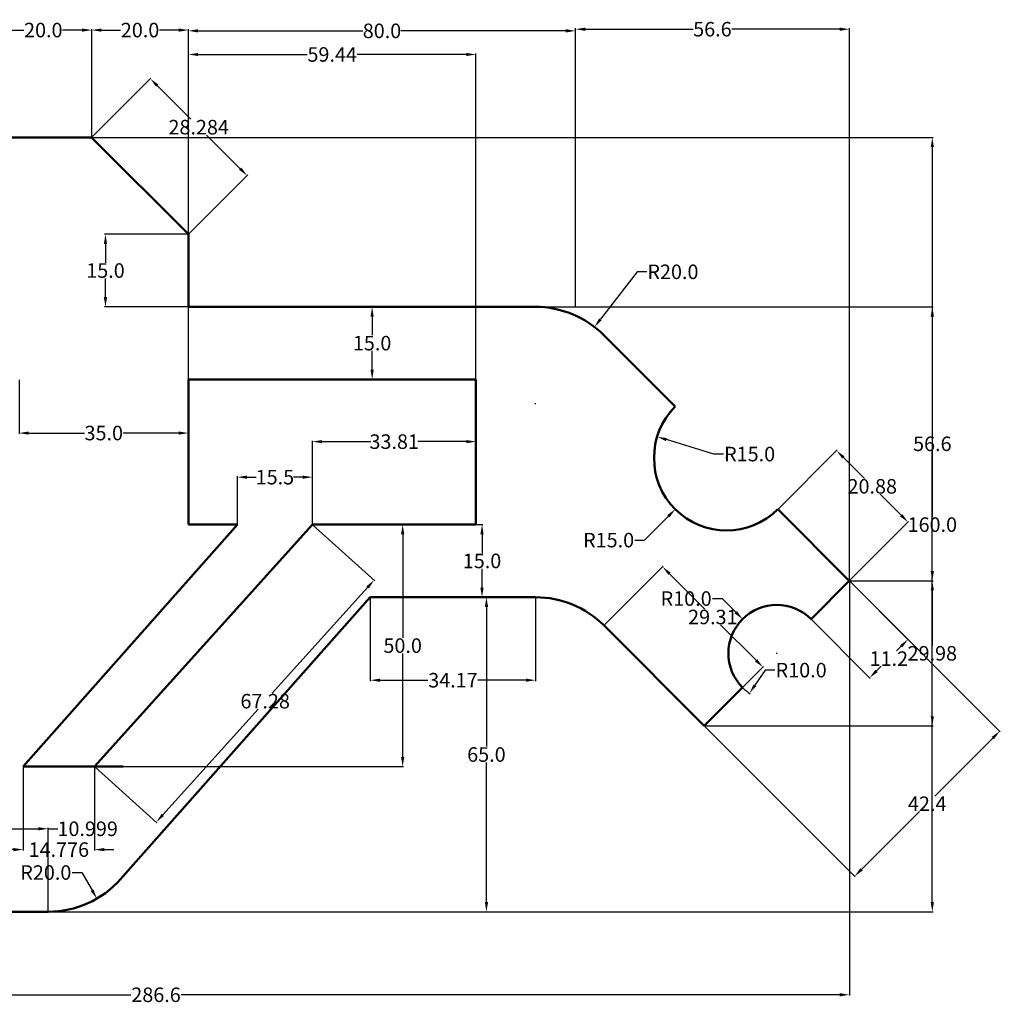
# Model space of a CAD drawing. Units: inches. Extents: x 142 to 482, y 54 to 269.
# Tile 2 of 2: x 279 to 482, y 54 to 258. Entities that reach past the tile are written whole.
import ezdxf

# ---------------------------------------------------------------- set-up
doc = ezdxf.new("R2010")
doc.units = ezdxf.units.IN
doc.header["$MEASUREMENT"] = 0
doc.layers.add('M-DIMS', color=2, linetype='Continuous', lineweight=25)
doc.layers.add('M-OUTL', color=7, linetype='Continuous', lineweight=50)
doc.styles.get("Standard").update_dxf_attribs({"font": 'arial.ttf'})
doc.dimstyles.get("Standard").update_dxf_attribs({"dimtxt": 3, "dimasz": 2, "dimexe": 0.18, "dimexo": 0.0625, "dimgap": 0.09, "dimtad": 0, "dimtih": 1, "dimtoh": 1, "dimdec": 1, "dimzin": 0, "dimdsep": 46, "dimtxsty": 'Standard', "dimcen": 0.09, "dimclrd": 1, "dimclre": 1, "dimadec": 0, "dimazin": 0, "dimtfac": 1, "dimtdec": 1, "dimtofl": 0, "dimtmove": 0, "dimatfit": 3, "dimfxl": 1, "dimtolj": 1, "dimtzin": 0, "dimarcsym": 0})

# ---------------------------------------------------------------- blocks, each defined once
blk = doc.blocks.new('*D9')
at = {"layer": 'Defpoints', "color": 0, "transparency": 16777216}
for p in [(293.74, 255.73), (273.74, 233.54), (293.74, 233.54)]:
    blk.add_point(p, dxfattribs=at)
at = {"layer": 'M-DIMS', "color": 0, "lineweight": -2, "transparency": 16777216}
for p, q in [((273.74, 233.6), (273.74, 255.91)), ((275.74, 255.73), (279.73, 255.73)), ((291.74, 255.73), (287.74, 255.73)), ((293.74, 233.6), (293.74, 255.91))]:
    blk.add_line(p, q, dxfattribs=at)
at = {"layer": 'M-DIMS', "color": 0, "transparency": 16777216}
for points in [[(275.74, 256.06), (275.74, 255.39), (273.74, 255.73)], [(291.74, 256.06), (291.74, 255.39), (293.74, 255.73)]]:
    blk.add_solid(points, dxfattribs=at)
at = {"layer": 'M-DIMS', "color": 0, "transparency": 16777216, "insert": (283.74, 255.73), "char_height": 3, "attachment_point": 5}
blk.add_mtext('\\A1;20.0', dxfattribs=at)
blk = doc.blocks.new('*D10')
at = {"layer": 'Defpoints', "color": 0, "transparency": 16777216}
for p in [(293.74, 255.73), (293.74, 233.54), (313.74, 213.54)]:
    blk.add_point(p, dxfattribs=at)
at = {"layer": 'M-DIMS', "color": 0, "lineweight": -2, "transparency": 16777216}
for p, q in [((293.74, 233.6), (293.74, 255.91)), ((295.74, 255.73), (299.73, 255.73)), ((311.74, 255.73), (307.74, 255.73)), ((313.74, 213.6), (313.74, 255.91))]:
    blk.add_line(p, q, dxfattribs=at)
at = {"layer": 'M-DIMS', "color": 0, "transparency": 16777216}
for points in [[(295.74, 256.06), (295.74, 255.39), (293.74, 255.73)], [(311.74, 256.06), (311.74, 255.39), (313.74, 255.73)]]:
    blk.add_solid(points, dxfattribs=at)
at = {"layer": 'M-DIMS', "color": 0, "transparency": 16777216, "insert": (303.74, 255.73), "char_height": 3, "attachment_point": 5}
blk.add_mtext('\\A1;20.0', dxfattribs=at)
blk = doc.blocks.new('*D11')
at = {"layer": 'Defpoints', "color": 0, "transparency": 16777216}
for p in [(351.7, 198.54), (336.38, 183.54), (351.7, 183.54)]:
    blk.add_point(p, dxfattribs=at)
at = {"layer": 'M-DIMS', "color": 0, "lineweight": -2, "transparency": 16777216}
for p, q in [((351.76, 198.54), (351.88, 198.54)), ((351.7, 196.54), (351.7, 192.66)), ((351.7, 185.54), (351.7, 189.42)), ((336.44, 183.54), (351.88, 183.54))]:
    blk.add_line(p, q, dxfattribs=at)
at = {"layer": 'M-DIMS', "color": 0, "transparency": 16777216}
for points in [[(351.37, 196.54), (352.03, 196.54), (351.7, 198.54)], [(351.37, 185.54), (352.03, 185.54), (351.7, 183.54)]]:
    blk.add_solid(points, dxfattribs=at)
at = {"layer": 'M-DIMS', "color": 0, "transparency": 16777216, "insert": (351.7, 191.04), "char_height": 3, "attachment_point": 5}
blk.add_mtext('\\A1;15.0', dxfattribs=at)
blk = doc.blocks.new('*D12')
at = {"layer": 'Defpoints', "color": 0, "transparency": 16777216}
for p in [(344.57, 153.54), (358.02, 153.54), (300.27, 103.54)]:
    blk.add_point(p, dxfattribs=at)
at = {"layer": 'M-DIMS', "color": 0, "lineweight": -2, "transparency": 16777216}
for p, q in [((344.63, 153.54), (358.2, 153.54)), ((358.02, 151.54), (358.02, 130.16)), ((358.02, 105.54), (358.02, 126.92)), ((300.34, 103.54), (358.2, 103.54))]:
    blk.add_line(p, q, dxfattribs=at)
at = {"layer": 'M-DIMS', "color": 0, "transparency": 16777216}
for points in [[(357.68, 151.54), (358.35, 151.54), (358.02, 153.54)], [(357.68, 105.54), (358.35, 105.54), (358.02, 103.54)]]:
    blk.add_solid(points, dxfattribs=at)
at = {"layer": 'M-DIMS', "color": 0, "transparency": 16777216, "insert": (358.02, 128.54), "char_height": 3, "attachment_point": 5}
blk.add_mtext('\\A1;50.0', dxfattribs=at)
blk = doc.blocks.new('*D13')
at = {"layer": 'Defpoints', "color": 0, "transparency": 16777216}
for p in [(372.53, 138.54), (375.33, 138.54), (284.73, 73.54)]:
    blk.add_point(p, dxfattribs=at)
at = {"layer": 'M-DIMS', "color": 0, "lineweight": -2, "transparency": 16777216}
for p, q in [((372.59, 138.54), (375.51, 138.54)), ((375.33, 136.54), (375.33, 107.66)), ((375.33, 75.54), (375.33, 104.42)), ((284.8, 73.54), (375.51, 73.54))]:
    blk.add_line(p, q, dxfattribs=at)
at = {"layer": 'M-DIMS', "color": 0, "transparency": 16777216}
for points in [[(375, 136.54), (375.67, 136.54), (375.33, 138.54)], [(375, 75.54), (375.67, 75.54), (375.33, 73.54)]]:
    blk.add_solid(points, dxfattribs=at)
at = {"layer": 'M-DIMS', "color": 0, "transparency": 16777216, "insert": (375.33, 106.04), "char_height": 3, "attachment_point": 5}
blk.add_mtext('\\A1;65.0', dxfattribs=at)
blk = doc.blocks.new('*D14')
at = {"layer": 'Defpoints', "color": 0, "transparency": 16777216}
for p in [(284.73, 93.54), (294.82, 76.27)]:
    blk.add_point(p, dxfattribs=at)
at = {"layer": 'M-DIMS', "color": 0, "lineweight": -2, "transparency": 16777216}
for p, q in [((289.68, 81.65), (291.68, 81.65)), ((291.68, 81.65), (293.81, 77.99))]:
    blk.add_line(p, q, dxfattribs=at)
at = {"layer": 'M-DIMS', "color": 0, "transparency": 16777216}
blk.add_solid([(294.1, 78.16), (293.52, 77.82), (294.82, 76.27)], dxfattribs=at)
at = {"layer": 'M-DIMS', "color": 0, "transparency": 16777216, "insert": (284.26, 81.65), "char_height": 3, "attachment_point": 5}
blk.add_mtext('\\A1;R20.0', dxfattribs=at)
blk = doc.blocks.new('*D15')
at = {"layer": 'Defpoints', "color": 0, "transparency": 16777216}
for p in [(393.74, 255.91), (393.74, 198.54), (450.34, 141.94)]:
    blk.add_point(p, dxfattribs=at)
at = {"layer": 'M-DIMS', "color": 0, "lineweight": -2, "transparency": 16777216}
for p, q in [((393.74, 198.6), (393.74, 256.09)), ((395.74, 255.91), (418.05, 255.91)), ((448.34, 255.91), (426.02, 255.91)), ((450.34, 142), (450.34, 256.09))]:
    blk.add_line(p, q, dxfattribs=at)
at = {"layer": 'M-DIMS', "color": 0, "transparency": 16777216}
for points in [[(395.74, 256.24), (395.74, 255.57), (393.74, 255.91)], [(448.34, 256.24), (448.34, 255.57), (450.34, 255.91)]]:
    blk.add_solid(points, dxfattribs=at)
at = {"layer": 'M-DIMS', "color": 0, "transparency": 16777216, "insert": (422.04, 255.91), "char_height": 3, "attachment_point": 5}
blk.add_mtext('\\A1;56.6', dxfattribs=at)
blk = doc.blocks.new('*D16')
at = {"layer": 'Defpoints', "color": 0, "transparency": 16777216}
for p in [(450.34, 141.94), (420.35, 111.96), (451.43, 80.88)]:
    blk.add_point(p, dxfattribs=at)
at = {"layer": 'M-DIMS', "color": 0, "lineweight": -2, "transparency": 16777216}
for p, q in [((450.38, 141.89), (481.54, 110.73)), ((420.4, 111.91), (451.56, 80.75)), ((480, 109.44), (468.02, 97.46)), ((452.85, 82.29), (464.83, 94.27))]:
    blk.add_line(p, q, dxfattribs=at)
at = {"layer": 'M-DIMS', "color": 0, "transparency": 16777216}
for points in [[(479.77, 109.68), (480.24, 109.21), (481.42, 110.86)], [(452.61, 82.53), (453.08, 82.06), (451.43, 80.88)]]:
    blk.add_solid(points, dxfattribs=at)
at = {"layer": 'M-DIMS', "color": 0, "transparency": 16777216, "insert": (466.43, 95.87), "char_height": 3, "attachment_point": 5}
blk.add_mtext('\\A1;42.4', dxfattribs=at)
blk = doc.blocks.new('*D17')
at = {"layer": 'Defpoints', "color": 0, "transparency": 16777216}
for p in [(397.67, 194.38), (385.45, 178.54)]:
    blk.add_point(p, dxfattribs=at)
at = {"layer": 'M-DIMS', "color": 0, "lineweight": -2, "transparency": 16777216}
for p, q in [((406.46, 205.78), (398.89, 195.96)), ((408.46, 205.78), (406.46, 205.78)), ((385.36, 178.54), (385.54, 178.54)), ((385.45, 178.45), (385.45, 178.63))]:
    blk.add_line(p, q, dxfattribs=at)
at = {"layer": 'M-DIMS', "color": 0, "transparency": 16777216}
blk.add_solid([(398.62, 196.16), (399.15, 195.76), (397.67, 194.38)], dxfattribs=at)
at = {"layer": 'M-DIMS', "color": 0, "transparency": 16777216, "insert": (413.88, 205.78), "char_height": 3, "attachment_point": 5}
blk.add_mtext('\\A1;R20.0', dxfattribs=at)
blk = doc.blocks.new('*D18')
at = {"layer": 'Defpoints', "color": 0, "transparency": 16777216}
for p in [(373.17, 153.54), (374.42, 138.54), (374.42, 138.54)]:
    blk.add_point(p, dxfattribs=at)
at = {"layer": 'M-DIMS', "color": 0, "lineweight": -2, "transparency": 16777216}
for p, q in [((373.23, 153.54), (374.6, 153.54)), ((374.42, 151.54), (374.42, 147.66)), ((374.42, 140.54), (374.42, 144.42)), ((374.48, 138.54), (374.6, 138.54))]:
    blk.add_line(p, q, dxfattribs=at)
at = {"layer": 'M-DIMS', "color": 0, "transparency": 16777216}
for points in [[(374.08, 151.54), (374.75, 151.54), (374.42, 153.54)], [(374.08, 140.54), (374.75, 140.54), (374.42, 138.54)]]:
    blk.add_solid(points, dxfattribs=at)
at = {"layer": 'M-DIMS', "color": 0, "transparency": 16777216, "insert": (374.42, 146.04), "char_height": 3, "attachment_point": 5}
blk.add_mtext('\\A1;15.0', dxfattribs=at)
blk = doc.blocks.new('*D19')
at = {"layer": 'Defpoints', "color": 0, "transparency": 16777216}
for p in [(339.36, 163.35), (323.86, 153.54), (339.36, 153.54)]:
    blk.add_point(p, dxfattribs=at)
at = {"layer": 'M-DIMS', "color": 0, "lineweight": -2, "transparency": 16777216}
for p, q in [((323.86, 153.6), (323.86, 163.53)), ((325.86, 163.35), (327.76, 163.35)), ((337.36, 163.35), (335.47, 163.35)), ((339.36, 153.6), (339.36, 163.53))]:
    blk.add_line(p, q, dxfattribs=at)
at = {"layer": 'M-DIMS', "color": 0, "transparency": 16777216}
for points in [[(325.86, 163.68), (325.86, 163.01), (323.86, 163.35)], [(337.36, 163.68), (337.36, 163.01), (339.36, 163.35)]]:
    blk.add_solid(points, dxfattribs=at)
at = {"layer": 'M-DIMS', "color": 0, "transparency": 16777216, "insert": (331.61, 163.35), "char_height": 3, "attachment_point": 5}
blk.add_mtext('\\A1;15.5', dxfattribs=at)
blk = doc.blocks.new('*D20')
at = {"layer": 'Defpoints', "color": 0, "transparency": 16777216}
for p in [(435.35, 126.95), (429.7, 118.69)]:
    blk.add_point(p, dxfattribs=at)
at = {"layer": 'M-DIMS', "color": 0, "lineweight": -2, "transparency": 16777216}
for p, q in [((432.97, 123.47), (430.83, 120.34)), ((434.97, 123.47), (432.97, 123.47))]:
    blk.add_line(p, q, dxfattribs=at)
blk.add_arc((435.35, 126.95), 10, 225.3581, 236.6689, dxfattribs=at)
at = {"layer": 'M-DIMS', "color": 0, "transparency": 16777216}
blk.add_solid([(430.55, 120.53), (431.1, 120.16), (429.7, 118.69)], dxfattribs=at)
at = {"layer": 'M-DIMS', "color": 0, "transparency": 16777216, "insert": (440.38, 123.47), "char_height": 3, "attachment_point": 5}
blk.add_mtext('\\A1;R10.0', dxfattribs=at)
blk = doc.blocks.new('*D21')
at = {"layer": 'Defpoints', "color": 0, "transparency": 16777216}
for p in [(410.62, 171.68), (424.96, 167.31)]:
    blk.add_point(p, dxfattribs=at)
at = {"layer": 'M-DIMS', "color": 0, "lineweight": -2, "transparency": 16777216}
for p, q in [((422.31, 168.12), (412.53, 171.1)), ((424.31, 168.12), (422.31, 168.12))]:
    blk.add_line(p, q, dxfattribs=at)
at = {"layer": 'M-DIMS', "color": 0, "transparency": 16777216}
blk.add_solid([(412.63, 171.42), (412.43, 170.78), (410.62, 171.68)], dxfattribs=at)
at = {"layer": 'M-DIMS', "color": 0, "transparency": 16777216, "insert": (429.73, 168.12), "char_height": 3, "attachment_point": 5}
blk.add_mtext('\\A1;R15.0', dxfattribs=at)
blk = doc.blocks.new('*D25')
at = {"layer": 'Defpoints', "color": 0, "transparency": 16777216}
for p in [(393.74, 255.57), (313.74, 213.54), (393.74, 198.54)]:
    blk.add_point(p, dxfattribs=at)
at = {"layer": 'M-DIMS', "color": 0, "lineweight": -2, "transparency": 16777216}
for p, q in [((313.74, 213.6), (313.74, 255.75)), ((315.74, 255.57), (349.75, 255.57)), ((391.74, 255.57), (357.72, 255.57)), ((393.74, 198.6), (393.74, 255.75))]:
    blk.add_line(p, q, dxfattribs=at)
at = {"layer": 'M-DIMS', "color": 0, "transparency": 16777216}
for points in [[(315.74, 255.91), (315.74, 255.24), (313.74, 255.57)], [(391.74, 255.91), (391.74, 255.24), (393.74, 255.57)]]:
    blk.add_solid(points, dxfattribs=at)
at = {"layer": 'M-DIMS', "color": 0, "transparency": 16777216, "insert": (353.74, 255.57), "char_height": 3, "attachment_point": 5}
blk.add_mtext('\\A1;80.0', dxfattribs=at)
blk = doc.blocks.new('*D26')
at = {"layer": 'Defpoints', "color": 0, "transparency": 16777216}
for p in [(278.74, 183.54), (313.74, 183.54), (313.74, 172.46)]:
    blk.add_point(p, dxfattribs=at)
at = {"layer": 'M-DIMS', "color": 0, "lineweight": -2, "transparency": 16777216}
for p, q in [((278.74, 183.48), (278.74, 172.28)), ((313.74, 183.48), (313.74, 172.28)), ((280.74, 172.46), (292.26, 172.46)), ((311.74, 172.46), (300.22, 172.46))]:
    blk.add_line(p, q, dxfattribs=at)
at = {"layer": 'M-DIMS', "color": 0, "transparency": 16777216}
for points in [[(280.74, 172.79), (280.74, 172.13), (278.74, 172.46)], [(311.74, 172.79), (311.74, 172.13), (313.74, 172.46)]]:
    blk.add_solid(points, dxfattribs=at)
at = {"layer": 'M-DIMS', "color": 0, "transparency": 16777216, "insert": (296.24, 172.46), "char_height": 3, "attachment_point": 5}
blk.add_mtext('\\A1;35.0', dxfattribs=at)
blk = doc.blocks.new('*D27')
at = {"layer": 'Defpoints', "color": 0, "transparency": 16777216}
for p in [(450.34, 141.94), (163.74, 93.54), (450.34, 56.39)]:
    blk.add_point(p, dxfattribs=at)
at = {"layer": 'M-DIMS', "color": 1, "lineweight": -2, "transparency": 16777216}
for p, q in [((450.34, 141.88), (450.34, 56.21)), ((163.74, 93.48), (163.74, 56.21)), ((165.74, 56.39), (301.86, 56.39)), ((448.34, 56.39), (312.21, 56.39))]:
    blk.add_line(p, q, dxfattribs=at)
at = {"layer": 'M-DIMS', "color": 1, "transparency": 16777216}
for points in [[(165.74, 56.72), (165.74, 56.06), (163.74, 56.39)], [(448.34, 56.72), (448.34, 56.06), (450.34, 56.39)]]:
    blk.add_solid(points, dxfattribs=at)
at = {"layer": 'M-DIMS', "color": 0, "transparency": 16777216, "insert": (307.04, 56.39), "char_height": 3, "attachment_point": 5}
blk.add_mtext('\\A1;286.6', dxfattribs=at)
blk = doc.blocks.new('*D28')
at = {"layer": 'Defpoints', "color": 0, "transparency": 16777216}
for p in [(293.74, 233.54), (467.49, 233.54), (284.73, 73.54)]:
    blk.add_point(p, dxfattribs=at)
at = {"layer": 'M-DIMS', "color": 1, "lineweight": -2, "transparency": 16777216}
for p, q in [((293.8, 233.54), (467.67, 233.54)), ((467.49, 231.54), (467.49, 155.16)), ((467.49, 75.54), (467.49, 151.92)), ((284.8, 73.54), (467.67, 73.54))]:
    blk.add_line(p, q, dxfattribs=at)
at = {"layer": 'M-DIMS', "color": 1, "transparency": 16777216}
for points in [[(467.15, 231.54), (467.82, 231.54), (467.49, 233.54)], [(467.15, 75.54), (467.82, 75.54), (467.49, 73.54)]]:
    blk.add_solid(points, dxfattribs=at)
at = {"layer": 'M-DIMS', "color": 0, "transparency": 16777216, "insert": (467.49, 153.54), "char_height": 3, "attachment_point": 5}
blk.add_mtext('\\A1;160.0', dxfattribs=at)
blk = doc.blocks.new('*D30')
at = {"layer": 'Defpoints', "color": 0, "transparency": 16777216}
for p in [(373.17, 250.69), (313.74, 183.54), (373.17, 183.54)]:
    blk.add_point(p, dxfattribs=at)
at = {"layer": 'M-DIMS', "color": 1, "lineweight": -2, "transparency": 16777216}
for p, q in [((313.74, 183.6), (313.74, 250.87)), ((315.74, 250.69), (338.31, 250.69)), ((371.17, 250.69), (348.6, 250.69)), ((373.17, 183.6), (373.17, 250.87))]:
    blk.add_line(p, q, dxfattribs=at)
at = {"layer": 'M-DIMS', "color": 1, "transparency": 16777216}
for points in [[(315.74, 251.02), (315.74, 250.36), (313.74, 250.69)], [(371.17, 251.02), (371.17, 250.36), (373.17, 250.69)]]:
    blk.add_solid(points, dxfattribs=at)
at = {"layer": 'M-DIMS', "color": 0, "transparency": 16777216, "insert": (343.45, 250.69), "char_height": 3, "attachment_point": 5}
blk.add_mtext('\\A1;59.44', dxfattribs=at)
blk = doc.blocks.new('*D31')
at = {"layer": 'Defpoints', "color": 0, "transparency": 16777216}
for p in [(296.59, 213.54), (313.74, 213.54), (313.74, 198.54)]:
    blk.add_point(p, dxfattribs=at)
at = {"layer": 'M-DIMS', "color": 1, "lineweight": -2, "transparency": 16777216}
for p, q in [((313.67, 213.54), (296.41, 213.54)), ((296.59, 211.54), (296.59, 207.66)), ((296.59, 200.54), (296.59, 204.42)), ((313.67, 198.54), (296.41, 198.54))]:
    blk.add_line(p, q, dxfattribs=at)
at = {"layer": 'M-DIMS', "color": 1, "transparency": 16777216}
for points in [[(296.25, 211.54), (296.92, 211.54), (296.59, 213.54)], [(296.25, 200.54), (296.92, 200.54), (296.59, 198.54)]]:
    blk.add_solid(points, dxfattribs=at)
at = {"layer": 'M-DIMS', "color": 0, "transparency": 16777216, "insert": (296.59, 206.04), "char_height": 3, "attachment_point": 5}
blk.add_mtext('\\A1;15.0', dxfattribs=at)
blk = doc.blocks.new('*D32')
at = {"layer": 'Defpoints', "color": 0, "transparency": 16777216}
for p in [(373.17, 170.69), (339.36, 153.54), (373.17, 153.54)]:
    blk.add_point(p, dxfattribs=at)
at = {"layer": 'M-DIMS', "color": 1, "lineweight": -2, "transparency": 16777216}
for p, q in [((339.36, 153.6), (339.36, 170.87)), ((341.36, 170.69), (351.41, 170.69)), ((371.17, 170.69), (361.13, 170.69)), ((373.17, 153.6), (373.17, 170.87))]:
    blk.add_line(p, q, dxfattribs=at)
at = {"layer": 'M-DIMS', "color": 1, "transparency": 16777216}
for points in [[(341.36, 171.02), (341.36, 170.36), (339.36, 170.69)], [(371.17, 171.02), (371.17, 170.36), (373.17, 170.69)]]:
    blk.add_solid(points, dxfattribs=at)
at = {"layer": 'M-DIMS', "color": 0, "transparency": 16777216, "insert": (356.27, 170.69), "char_height": 3, "attachment_point": 5}
blk.add_mtext('\\A1;33.81', dxfattribs=at)
blk = doc.blocks.new('*D33')
at = {"layer": 'Defpoints', "color": 0, "transparency": 16777216}
for p in [(435.57, 156.7), (462.46, 154.07), (450.34, 141.94)]:
    blk.add_point(p, dxfattribs=at)
at = {"layer": 'M-DIMS', "color": 1, "lineweight": -2, "transparency": 16777216}
for p, q in [((435.62, 156.75), (447.83, 168.96)), ((449.11, 167.42), (453.46, 163.07)), ((461.05, 155.48), (456.7, 159.83)), ((450.38, 141.98), (462.59, 154.19))]:
    blk.add_line(p, q, dxfattribs=at)
at = {"layer": 'M-DIMS', "color": 1, "transparency": 16777216}
for points in [[(449.35, 167.65), (448.88, 167.18), (447.7, 168.83)], [(461.28, 155.72), (460.81, 155.24), (462.46, 154.07)]]:
    blk.add_solid(points, dxfattribs=at)
at = {"layer": 'M-DIMS', "color": 0, "transparency": 16777216, "insert": (455.08, 161.45), "char_height": 3, "attachment_point": 5}
blk.add_mtext('\\A1;20.88', dxfattribs=at)
blk = doc.blocks.new('*D34')
at = {"layer": 'Defpoints', "color": 0, "transparency": 16777216}
for p in [(450.34, 141.94), (442.42, 134.02), (454.54, 121.89)]:
    blk.add_point(p, dxfattribs=at)
at = {"layer": 'M-DIMS', "color": 1, "lineweight": -2, "transparency": 16777216}
for p, q in [((450.38, 141.89), (462.59, 129.68)), ((442.46, 133.98), (454.67, 121.77)), ((461.05, 128.4), (460.1, 127.45)), ((455.96, 123.31), (456.91, 124.26))]:
    blk.add_line(p, q, dxfattribs=at)
at = {"layer": 'M-DIMS', "color": 1, "transparency": 16777216}
for points in [[(460.81, 128.63), (461.28, 128.16), (462.46, 129.81)], [(455.72, 123.54), (456.19, 123.07), (454.54, 121.89)]]:
    blk.add_solid(points, dxfattribs=at)
at = {"layer": 'M-DIMS', "color": 0, "transparency": 16777216, "insert": (458.5, 125.85), "char_height": 3, "attachment_point": 5}
blk.add_mtext('\\A1;11.2', dxfattribs=at)
blk = doc.blocks.new('*D35')
at = {"layer": 'Defpoints', "color": 0, "transparency": 16777216}
for p in [(339.36, 153.54), (294.34, 103.54), (307.09, 92.06)]:
    blk.add_point(p, dxfattribs=at)
at = {"layer": 'M-DIMS', "color": 1, "lineweight": -2, "transparency": 16777216}
for p, q in [((339.41, 153.5), (352.24, 141.94)), ((350.77, 140.58), (331.06, 118.69)), ((308.43, 93.55), (328.14, 115.44)), ((294.39, 103.5), (307.22, 91.94))]:
    blk.add_line(p, q, dxfattribs=at)
at = {"layer": 'M-DIMS', "color": 1, "transparency": 16777216}
for points in [[(350.52, 140.8), (351.02, 140.35), (352.11, 142.06)], [(308.18, 93.77), (308.67, 93.33), (307.09, 92.06)]]:
    blk.add_solid(points, dxfattribs=at)
at = {"layer": 'M-DIMS', "color": 0, "transparency": 16777216, "insert": (329.6, 117.06), "char_height": 3, "attachment_point": 5}
blk.add_mtext('\\A1;67.28', dxfattribs=at)
blk = doc.blocks.new('*D36')
at = {"layer": 'Defpoints', "color": 0, "transparency": 16777216}
for p in [(279.57, 103.54), (294.34, 103.54), (279.57, 86.39)]:
    blk.add_point(p, dxfattribs=at)
at = {"layer": 'M-DIMS', "color": 1, "lineweight": -2, "transparency": 16777216}
for p, q in [((279.57, 103.48), (279.57, 86.21)), ((294.34, 103.48), (294.34, 86.21)), ((277.57, 86.39), (275.57, 86.39)), ((296.34, 86.39), (298.34, 86.39))]:
    blk.add_line(p, q, dxfattribs=at)
at = {"layer": 'M-DIMS', "color": 1, "transparency": 16777216}
for points in [[(277.57, 86.72), (277.57, 86.06), (279.57, 86.39)], [(296.34, 86.72), (296.34, 86.06), (294.34, 86.39)]]:
    blk.add_solid(points, dxfattribs=at)
at = {"layer": 'M-DIMS', "color": 0, "transparency": 16777216, "insert": (286.95, 86.39), "char_height": 3, "attachment_point": 5}
blk.add_mtext('\\A1;14.776', dxfattribs=at)
blk = doc.blocks.new('*D37')
at = {"layer": 'Defpoints', "color": 0, "transparency": 16777216}
for p in [(284.73, 90.69), (273.74, 73.54), (284.73, 73.54)]:
    blk.add_point(p, dxfattribs=at)
at = {"layer": 'M-DIMS', "color": 1, "lineweight": -2, "transparency": 16777216}
for p, q in [((273.74, 73.6), (273.74, 90.87)), ((275.74, 90.69), (282.73, 90.69)), ((284.73, 73.6), (284.73, 90.87)), ((284.73, 90.69), (286.73, 90.69))]:
    blk.add_line(p, q, dxfattribs=at)
at = {"layer": 'M-DIMS', "color": 1, "transparency": 16777216}
for points in [[(275.74, 91.02), (275.74, 90.36), (273.74, 90.69)], [(282.73, 91.02), (282.73, 90.36), (284.73, 90.69)]]:
    blk.add_solid(points, dxfattribs=at)
at = {"layer": 'M-DIMS', "color": 0, "transparency": 16777216, "insert": (292.91, 90.69), "char_height": 3, "attachment_point": 5}
blk.add_mtext('\\A1;10.999', dxfattribs=at)
blk = doc.blocks.new('*D38')
at = {"layer": 'Defpoints', "color": 0, "transparency": 16777216}
for p in [(351.32, 138.54), (385.49, 138.54), (351.32, 121.39)]:
    blk.add_point(p, dxfattribs=at)
at = {"layer": 'M-DIMS', "color": 1, "lineweight": -2, "transparency": 16777216}
for p, q in [((351.32, 138.48), (351.32, 121.21)), ((385.49, 138.48), (385.49, 121.21)), ((353.32, 121.39), (363.25, 121.39)), ((383.49, 121.39), (373.56, 121.39))]:
    blk.add_line(p, q, dxfattribs=at)
at = {"layer": 'M-DIMS', "color": 1, "transparency": 16777216}
for points in [[(353.32, 121.72), (353.32, 121.06), (351.32, 121.39)], [(383.49, 121.72), (383.49, 121.06), (385.49, 121.39)]]:
    blk.add_solid(points, dxfattribs=at)
at = {"layer": 'M-DIMS', "color": 0, "transparency": 16777216, "insert": (368.41, 121.39), "char_height": 3, "attachment_point": 5}
blk.add_mtext('\\A1;34.17', dxfattribs=at)
blk = doc.blocks.new('*D39')
at = {"layer": 'Defpoints', "color": 0, "transparency": 16777216}
for p in [(385.45, 198.54), (450.34, 141.94), (467.49, 141.94)]:
    blk.add_point(p, dxfattribs=at)
at = {"layer": 'M-DIMS', "color": 1, "lineweight": -2, "transparency": 16777216}
for p, q in [((385.51, 198.54), (467.67, 198.54)), ((467.49, 196.54), (467.49, 171.86)), ((467.49, 143.94), (467.49, 168.62)), ((450.4, 141.94), (467.67, 141.94))]:
    blk.add_line(p, q, dxfattribs=at)
at = {"layer": 'M-DIMS', "color": 1, "transparency": 16777216}
for points in [[(467.15, 196.54), (467.82, 196.54), (467.49, 198.54)], [(467.15, 143.94), (467.82, 143.94), (467.49, 141.94)]]:
    blk.add_solid(points, dxfattribs=at)
at = {"layer": 'M-DIMS', "color": 0, "transparency": 16777216, "insert": (467.49, 170.24), "char_height": 3, "attachment_point": 5}
blk.add_mtext('\\A1;56.6', dxfattribs=at)
blk = doc.blocks.new('*D40')
at = {"layer": 'Defpoints', "color": 0, "transparency": 16777216}
for p in [(450.34, 141.94), (467.49, 141.94), (420.35, 111.96)]:
    blk.add_point(p, dxfattribs=at)
at = {"layer": 'M-DIMS', "color": 1, "lineweight": -2, "transparency": 16777216}
for p, q in [((450.4, 141.94), (467.67, 141.94)), ((467.49, 139.94), (467.49, 128.57)), ((467.49, 113.96), (467.49, 125.33)), ((420.42, 111.96), (467.67, 111.96))]:
    blk.add_line(p, q, dxfattribs=at)
at = {"layer": 'M-DIMS', "color": 1, "transparency": 16777216}
for points in [[(467.15, 139.94), (467.82, 139.94), (467.49, 141.94)], [(467.15, 113.96), (467.82, 113.96), (467.49, 111.96)]]:
    blk.add_solid(points, dxfattribs=at)
at = {"layer": 'M-DIMS', "color": 0, "transparency": 16777216, "insert": (467.49, 126.95), "char_height": 3, "attachment_point": 5}
blk.add_mtext('\\A1;29.98', dxfattribs=at)
blk = doc.blocks.new('*D44')
at = {"layer": 'Defpoints', "color": 0, "transparency": 16777216}
for p in [(399.63, 132.68), (432.48, 124.08), (420.35, 111.96)]:
    blk.add_point(p, dxfattribs=at)
at = {"layer": 'M-DIMS', "color": 1, "lineweight": -2, "transparency": 16777216}
for p, q in [((399.68, 132.73), (411.89, 144.94)), ((413.17, 143.39), (420.5, 136.07)), ((431.07, 125.5), (423.74, 132.82)), ((420.4, 112), (432.61, 124.21))]:
    blk.add_line(p, q, dxfattribs=at)
at = {"layer": 'M-DIMS', "color": 1, "transparency": 16777216}
for points in [[(413.41, 143.63), (412.94, 143.16), (411.76, 144.81)], [(431.3, 125.73), (430.83, 125.26), (432.48, 124.08)]]:
    blk.add_solid(points, dxfattribs=at)
at = {"layer": 'M-DIMS', "color": 0, "transparency": 16777216, "insert": (422.12, 134.45), "char_height": 3, "attachment_point": 5}
blk.add_mtext('\\A1;29.31', dxfattribs=at)
blk = doc.blocks.new('*D46')
at = {"layer": 'Defpoints', "color": 0, "transparency": 16777216}
for p in [(293.74, 233.54), (325.86, 225.67), (313.74, 213.54)]:
    blk.add_point(p, dxfattribs=at)
at = {"layer": 'M-DIMS', "color": 1, "lineweight": -2, "transparency": 16777216}
for p, q in [((293.78, 233.58), (305.99, 245.79)), ((307.28, 244.25), (314.24, 237.29)), ((324.45, 227.08), (317.48, 234.04)), ((313.78, 213.58), (325.99, 225.79))]:
    blk.add_line(p, q, dxfattribs=at)
at = {"layer": 'M-DIMS', "color": 1, "transparency": 16777216}
for points in [[(307.51, 244.49), (307.04, 244.02), (305.86, 245.67)], [(324.68, 227.32), (324.21, 226.84), (325.86, 225.67)]]:
    blk.add_solid(points, dxfattribs=at)
at = {"layer": 'M-DIMS', "color": 0, "transparency": 16777216, "insert": (315.86, 235.67), "char_height": 3, "attachment_point": 5}
blk.add_mtext('\\A1;28.284', dxfattribs=at)
blk = doc.blocks.new('*D48')
at = {"layer": 'Defpoints', "color": 0, "transparency": 16777216}
for p in [(424.96, 167.31), (414.36, 156.7)]:
    blk.add_point(p, dxfattribs=at)
at = {"layer": 'M-DIMS', "color": 1, "lineweight": -2, "transparency": 16777216}
for p, q in [((424.87, 167.31), (425.05, 167.31)), ((424.96, 167.22), (424.96, 167.4)), ((407.99, 150.34), (412.94, 155.29)), ((405.99, 150.34), (407.99, 150.34))]:
    blk.add_line(p, q, dxfattribs=at)
at = {"layer": 'M-DIMS', "color": 1, "transparency": 16777216}
blk.add_solid([(412.71, 155.52), (413.18, 155.05), (414.36, 156.7)], dxfattribs=at)
at = {"layer": 'M-DIMS', "color": 0, "transparency": 16777216, "insert": (400.58, 150.34), "char_height": 3, "attachment_point": 5}
blk.add_mtext('\\A1;R15.0', dxfattribs=at)
blk = doc.blocks.new('*D49')
at = {"layer": 'Defpoints', "color": 0, "transparency": 16777216}
for p in [(428.27, 134.02), (435.35, 126.95)]:
    blk.add_point(p, dxfattribs=at)
at = {"layer": 'M-DIMS', "color": 1, "lineweight": -2, "transparency": 16777216}
for p, q in [((422.03, 138.26), (424.03, 138.26)), ((424.03, 138.26), (426.86, 135.43)), ((435.26, 126.95), (435.44, 126.95)), ((435.35, 126.86), (435.35, 127.04))]:
    blk.add_line(p, q, dxfattribs=at)
at = {"layer": 'M-DIMS', "color": 1, "transparency": 16777216}
blk.add_solid([(427.1, 135.67), (426.62, 135.2), (428.27, 134.02)], dxfattribs=at)
at = {"layer": 'M-DIMS', "color": 0, "transparency": 16777216, "insert": (416.61, 138.26), "char_height": 3, "attachment_point": 5}
blk.add_mtext('\\A1;R10.0', dxfattribs=at)

msp = doc.modelspace()

# ---------------------------------------------------------------- linework, layer by layer
at = {"layer": 'M-OUTL'}
for p, q in [((273.7359, 233.539), (293.7359, 233.539)), ((313.7359, 213.539), (293.7359, 233.539)), ((313.7359, 213.539), (313.7359, 198.539)), ((313.7359, 198.539), (385.4516, 198.539)), ((399.5937, 192.6811), (414.3582, 177.9166)), ((313.7359, 183.539), (373.1715, 183.539)), ((313.7359, 183.539), (313.7359, 153.539)), ((373.1715, 183.539), (373.1715, 153.539)), ((435.5714, 156.7034), (450.3359, 141.939)), ((279.566, 103.539), (323.8626, 153.539)), ((339.3626, 153.539), (294.3424, 103.539)), ((313.7359, 153.539), (323.8626, 153.539)), ((339.3626, 153.539), (373.1715, 153.539)), ((450.3359, 141.939), (442.4163, 134.0194)), ((299.7048, 80.2765), (351.3213, 138.539)), ((351.3213, 138.539), (385.4889, 138.539)), ((399.6311, 132.6811), (420.3545, 111.9576)), ((428.2741, 119.8772), (420.3545, 111.9576)), ((300.2739, 103.539), (279.566, 103.539)), ((273.7359, 73.539), (284.7346, 73.539))]:
    msp.add_line(p, q, dxfattribs=at)
for centre, radius, start, end in [((385.4516, 178.539), 20, 45, 90), ((424.9648, 167.31), 15, 135, 315), ((385.4889, 118.539), 20, 45, 90), ((435.3452, 126.9483), 10, 45, 225), ((284.7346, 93.539), 20, 270, 318.461294)]:
    msp.add_arc(centre, radius, start, end, dxfattribs=at)

# ---------------------------------------------------------------- dimensions: what is measured, and where the dimension line sits
at = {"layer": 'M-DIMS'}
for base, p1, p2, override, picture, middle in [((293.7359, 255.7265), (273.7359, 233.539), (293.7359, 233.539), {"dimclrd": 0, "dimclre": 0, "dimclrt": 0}, '*D9', (283.7359, 255.7265)), ((293.7359, 255.7265), (313.7359, 213.539), (293.7359, 233.539), {"dimclrd": 0, "dimclre": 0, "dimclrt": 0}, '*D10', (303.7359, 255.7265)), ((393.7359, 255.5731), (313.7359, 213.539), (393.7359, 198.539), {"dimclrd": 0, "dimclre": 0, "dimclrt": 0}, '*D25', (353.7359, 255.5731)), ((393.7359, 255.9065), (450.3359, 141.939), (393.7359, 198.539), {"dimclrd": 0, "dimclre": 0, "dimclrt": 0}, '*D15', (422.0359, 255.9065)), ((373.1715, 250.689), (313.7359, 183.539), (373.1715, 183.539), {"dimdec": 2, "dimlfac": 1, "dimrnd": 0, "dimzin": 0, "dimdsep": 46, "dimlunit": 2}, '*D30', (343.4537, 250.689)), ((313.7359, 172.4595), (278.7359, 183.539), (313.7359, 183.539), {"dimclrd": 0, "dimclre": 0, "dimclrt": 0}, '*D26', (296.2359, 172.4595)), ((373.1715, 170.689), (339.3626, 153.539), (373.1715, 153.539), {"dimdec": 2, "dimlfac": 1, "dimrnd": 0, "dimzin": 0, "dimdsep": 46, "dimlunit": 2}, '*D32', (356.2671, 170.689)), ((339.3626, 163.3466), (323.8626, 153.539), (339.3626, 153.539), {"dimclrd": 0, "dimclre": 0, "dimclrt": 0}, '*D19', (331.6126, 163.3466)), ((450.3359, 56.389), (163.7359, 93.539), (450.3359, 141.939), {"dimdec": 1, "dimlfac": 1, "dimrnd": 0, "dimzin": 0, "dimdsep": 46, "dimlunit": 2}, '*D27', (307.0359, 56.389))]:
    dim = msp.add_linear_dim(base=base, p1=p1, p2=p2, dimstyle='Standard', override=override, dxfattribs=at)
    dim.commit()
    dim.dimension.update_dxf_attribs({"geometry": picture, "text_midpoint": middle})
for base, p1, p2, angle, override, picture, middle in [((325.8627, 225.6659), (293.7359, 233.539), (313.7359, 213.539), 315, {"dimdec": 3, "dimlfac": 1, "dimrnd": 0, "dimzin": 0, "dimdsep": 46, "dimlunit": 2}, '*D46', (315.8627, 235.6659)), ((467.4859, 233.539), (284.7346, 73.539), (293.7359, 233.539), 90, {"dimdec": 1, "dimlfac": 1, "dimrnd": 0, "dimzin": 0, "dimdsep": 46, "dimlunit": 2}, '*D28', (467.4859, 153.539)), ((296.5859, 213.539), (313.7359, 198.539), (313.7359, 213.539), 90, {"dimdec": 1, "dimlfac": 1, "dimrnd": 0, "dimzin": 0, "dimdsep": 46, "dimlunit": 2}, '*D31', (296.5859, 206.039)), ((351.7014, 183.539), (351.7014, 198.539), (336.3772, 183.539), 90, {"dimclrd": 0, "dimclre": 0, "dimclrt": 0}, '*D11', (351.7014, 191.039)), ((467.4859, 141.939), (385.4516, 198.539), (450.3359, 141.939), 90, {"dimdec": 1, "dimlfac": 1, "dimrnd": 0, "dimzin": 0, "dimdsep": 46, "dimlunit": 2}, '*D39', (467.4859, 170.239)), ((462.4627, 154.0659), (435.5714, 156.7034), (450.3359, 141.939), 315, {"dimdec": 2, "dimlfac": 1, "dimrnd": 0, "dimzin": 0, "dimdsep": 46, "dimlunit": 2}, '*D33', (455.0805, 161.4481)), ((307.0873, 92.0634), (339.3626, 153.539), (294.3424, 103.539), 228, {"dimdec": 2, "dimlfac": 1, "dimrnd": 0, "dimzin": 0, "dimdsep": 46, "dimlunit": 2}, '*D35', (329.5974, 117.0634)), ((358.0166, 153.539), (300.2739, 103.539), (344.5704, 153.539), 90, {"dimclrd": 0, "dimclre": 0, "dimclrt": 0}, '*D12', (358.0166, 128.539)), ((374.4153, 138.539), (373.1715, 153.539), (374.4153, 138.539), 90, {"dimclrd": 0, "dimclre": 0, "dimclrt": 0}, '*D18', (374.4153, 146.039)), ((432.4814, 124.0845), (399.6311, 132.6811), (420.3545, 111.9576), 315, {"dimdec": 2, "dimlfac": 1, "dimrnd": 0, "dimzin": 0, "dimdsep": 46, "dimlunit": 2}, '*D44', (422.1197, 134.4463)), ((467.4859, 141.939), (420.3545, 111.9576), (450.3359, 141.939), 90, {"dimdec": 2, "dimlfac": 1, "dimrnd": 0, "dimzin": 0, "dimdsep": 46, "dimlunit": 2}, '*D40', (467.4859, 126.9483)), ((454.5432, 121.8925), (450.3359, 141.939), (442.4163, 134.0194), 225, {"dimdec": 1, "dimlfac": 1, "dimrnd": 0, "dimzin": 0, "dimdsep": 46, "dimlunit": 2}, '*D34', (458.503, 125.8523)), ((375.3332, 138.539), (284.7346, 73.539), (372.5286, 138.539), 90, {"dimclrd": 0, "dimclre": 0, "dimclrt": 0}, '*D13', (375.3332, 106.039)), ((351.3213, 121.389), (385.4889, 138.539), (351.3213, 138.539), 180, {"dimdec": 2, "dimlfac": 1, "dimrnd": 0, "dimzin": 0, "dimdsep": 46, "dimlunit": 2}, '*D38', (368.4051, 121.389)), ((279.566, 86.389), (294.3424, 103.539), (279.566, 103.539), 180, {"dimdec": 3, "dimlfac": 1, "dimrnd": 0, "dimzin": 0, "dimdsep": 46, "dimlunit": 2}, '*D36', (286.9542, 86.389)), ((284.7346, 90.689), (273.7359, 73.539), (284.7346, 73.539), 0, {"dimdec": 3, "dimlfac": 1, "dimrnd": 0, "dimzin": 0, "dimdsep": 46, "dimlunit": 2}, '*D37', (292.9137, 90.689))]:
    dim = msp.add_linear_dim(base=base, p1=p1, p2=p2, angle=angle, dimstyle='Standard', override=override, dxfattribs=at)
    dim.commit()
    dim.dimension.update_dxf_attribs({"geometry": picture, "text_midpoint": middle})
for center, mpoint, override, picture, middle in [((385.4516, 178.539), (397.6652, 194.3765), {"dimclrd": 0, "dimclre": 0, "dimclrt": 0}, '*D17', (413.8764, 205.7803)), ((424.9648, 167.31), (410.616, 171.6817), {"dimclrd": 0, "dimclre": 0, "dimclrt": 0}, '*D21', (429.7283, 168.1184)), ((424.9648, 167.31), (414.3583, 156.7033), {"dimdec": 1, "dimlfac": 1, "dimrnd": 0, "dimzin": 0, "dimdsep": 46, "dimlunit": 2}, '*D48', (400.5777, 150.3393)), ((435.3452, 126.9483), (428.2739, 134.0191), {"dimdec": 1, "dimlfac": 1, "dimrnd": 0, "dimzin": 0, "dimdsep": 46, "dimlunit": 2}, '*D49', (416.6143, 138.2616)), ((435.3452, 126.9483), (429.701, 118.6935), {"dimclrd": 0, "dimclre": 0, "dimclrt": 0}, '*D20', (440.3818, 123.4672)), ((284.7346, 93.539), (294.8155, 76.2654), {"dimclrd": 0, "dimclre": 0, "dimclrt": 0}, '*D14', (284.2586, 81.646))]:
    dim = msp.add_radius_dim(center=center, mpoint=mpoint, dimstyle='Standard', override=override, dxfattribs=at)
    dim.commit()
    dim.dimension.update_dxf_attribs({"geometry": picture, "text_midpoint": middle, "dimtype": 164})
dim = msp.add_aligned_dim(p1=(450.3359, 141.939), p2=(420.3545, 111.9576), distance=43.9539, dimstyle='Standard', override={"dimclrd": 0, "dimclre": 0, "dimclrt": 0}, dxfattribs=at)
dim.commit()
dim.dimension.update_dxf_attribs({"geometry": '*D16', "text_midpoint": (466.4253, 95.8682)})

doc.saveas('drawing.dxf')
